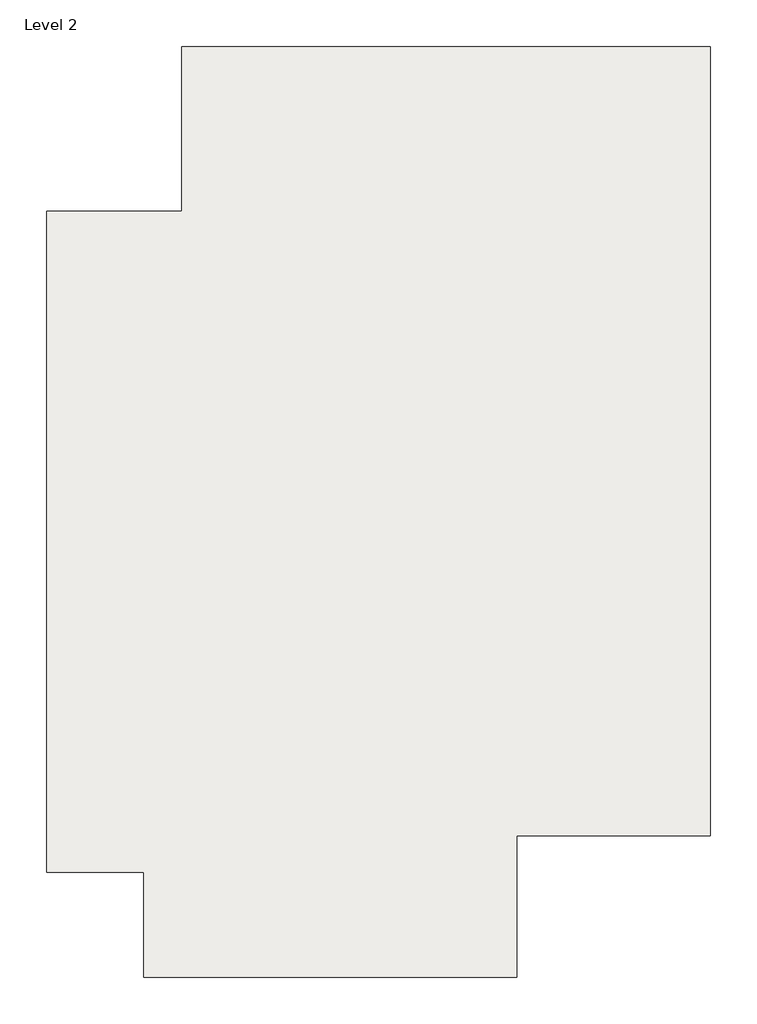
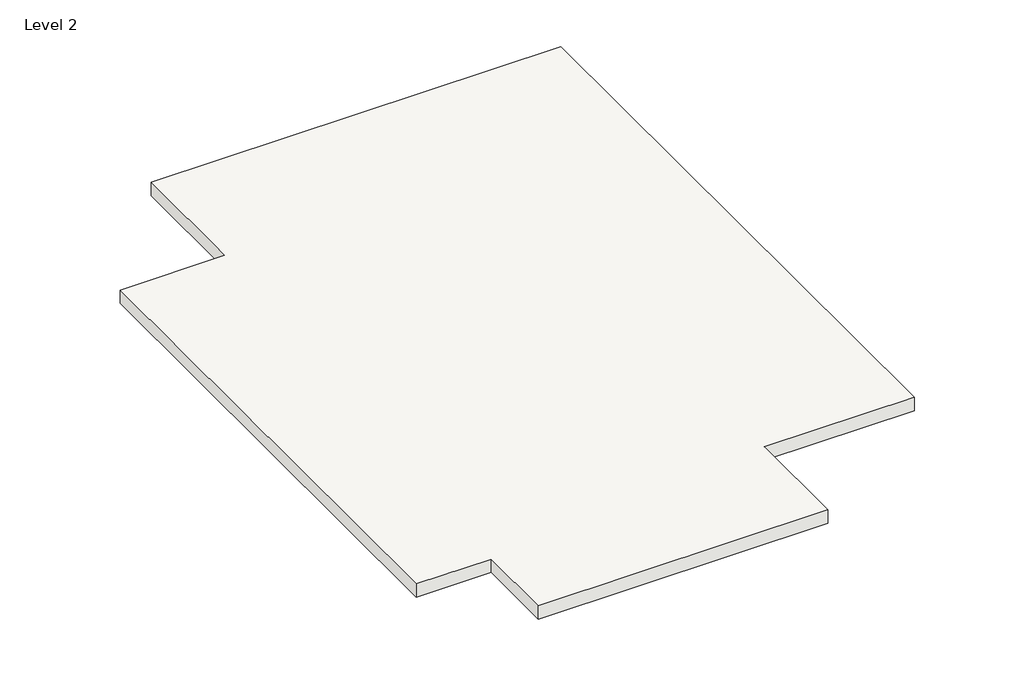
# One storey: 1 roof.
"""IFC4 building model written with IfcOpenShell, lengths in millimetres."""

from ifc_helpers import new_model, si_unit, frame, origin, place, context, project, spatial, polyline, outline, extrude, element, save

model = new_model("IFC4")

# Units and contexts
model_context = context("Model", 3, world=origin())
ifc_project = project(units=[si_unit("LENGTHUNIT", "METRE", prefix="MILLI")], contexts=[model_context])

# Site, building, storey
site = spatial("IfcSite", under=ifc_project)
building = spatial("IfcBuilding", under=site)
storey = spatial("IfcBuildingStorey", under=building, Name="Level 2", Elevation=3048.0)

# Roof
placement = place(None, origin())
element("IfcRoof", 1, ObjectType="Generic - 12\"", at=placement, inside=storey, context=model_context, shape_type="SweptSolid", body=[
    extrude(outline(polyline([(-15796.5727047, 7210.2673329), (-13543.8159934, 7210.2673329), (-13543.8159934, 9953.4673329), (-4730.0159934, 9953.4673329), (-4730.0159934, -3203.7326671), (-7955.8159934, -3203.7326671), (-7955.8159934, -5565.9326671), (-14178.8159934, -5565.9326671), (-14178.8159934, -3813.3326671), (-15796.5727047, -3813.3326671), (-15796.5727047, 7210.2673329)])), frame((0.0, 0.0, 3048.0), z_axis=(0.0, 0.0, 1.0), x_axis=(1.0, 0.0, 0.0)), (0.0, 0.0, 1.0), 304.8),
])

save(model, "model.ifc")

# Revit data of these elements
# Type "Generic - 12\""
#   Assembly Code = "B1020"
#   Layers, outside or top first: 1' - 0" "Brick, Soldier Course" (function 1)
# Element 1 (IfcRoof, "Generic - 12\"")
#   built-in parameter 1001705 = 11 (stored number, unit not read)
#   built-in parameter 1001710 = 33615
#   Phase Created = New Construction
#   Materials on its faces: "Brick, Soldier Course"
# Materials
#   "Brick, Soldier Course": class "Masonry", colour RGB 170 98 104, transparency 0, Description = "Common brick soldier coursed", Cost = 0
